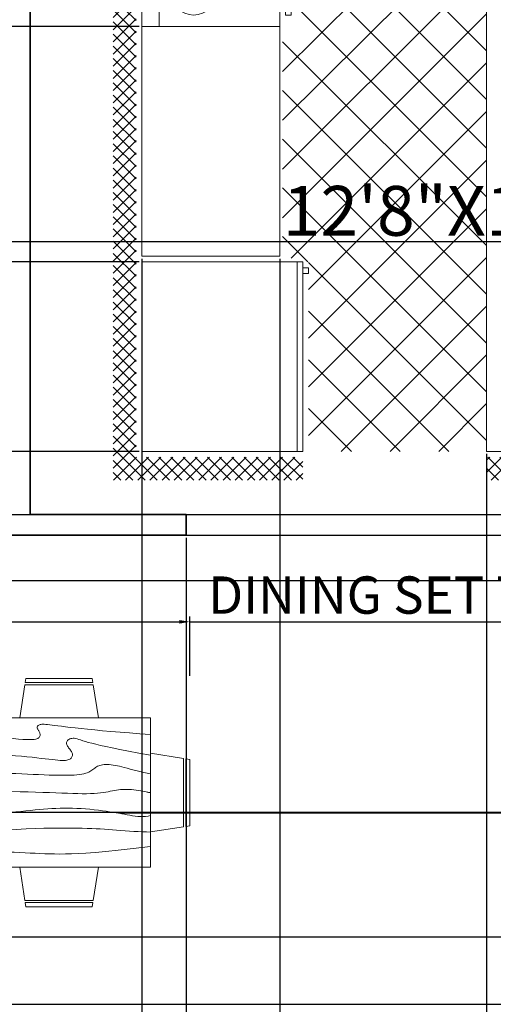
# Model space of a CAD drawing. Units: inches. Extents: x 3542 to 4275, y 1005 to 1722.
# Tile 4 of 6: x 4018 to 4132, y 1330 to 1568. Entities that reach past the tile are written whole.
import ezdxf

# ---------------------------------------------------------------- set-up
doc = ezdxf.new("R2010")
doc.units = ezdxf.units.IN
doc.layers.get('0').update_dxf_attribs({"color": 211})
for name, color, linetype, lineweight in [('A-ANNO-DIMS', 2, 'Continuous', 18), ('A-AREA-IDEN', 7, 'Continuous', 25), ('A-FLOR-FIXT', 9, 'Continuous', 18), ('A-FURN', 8, 'Continuous', 18), ('wall', 7, 'Continuous', 35)]:
    doc.layers.add(name, color=color, linetype=linetype, lineweight=lineweight)
doc.styles.get("Standard").update_dxf_attribs({"font": 'arial.ttf'})
doc.dimstyles.new('ISO-25', dxfattribs={"dimtxt": 9, "dimasz": 2.5, "dimexe": 1.25, "dimexo": 0.625, "dimtad": 1, "dimdec": 1, "dimlunit": 4, "dimtxsty": 'Standard', "dimcen": 2.5, "dimadec": 0, "dimazin": 0, "dimtfac": 1, "dimtdec": 1, "dimtmove": 0, "dimatfit": 3, "dimfxl": 1, "dimarcsym": 0})

# ---------------------------------------------------------------- blocks, each defined once
blk = doc.blocks.new('Kitchen Layout - 7 x 8 ft')
for p, q in [((-5, 81.32), (2.68, 89)), ((-5, 83.44), (0.56, 89)), ((-5, 85.56), (-1.56, 89)), ((-5, 87.68), (-3.68, 89)), ((-1, 84.97), (-5, 88.97)), ((1.09, 85), (-2.91, 89)), ((3.21, 85), (-0.79, 89)), ((0.81, 85), (4.81, 89)), ((5.34, 85), (1.34, 89)), ((2.93, 85), (6.93, 89)), ((7.46, 85), (3.46, 89)), ((5.05, 85), (9.05, 89)), ((9.58, 85), (5.58, 89)), ((7.17, 85), (11.17, 89)), ((11.7, 85), (7.7, 89)), ((9.29, 85), (13.29, 89)), ((13.82, 85), (9.82, 89)), ((11.41, 85), (15.41, 89)), ((15.94, 85), (11.94, 89)), ((13.53, 85), (17.53, 89)), ((18.06, 85), (14.06, 89)), ((15.65, 85), (19.65, 89)), ((20.18, 85), (16.18, 89)), ((17.78, 85), (21.78, 89)), ((22.31, 85), (18.31, 89)), ((19.9, 85), (23.9, 89)), ((24.43, 85), (20.43, 89)), ((22.02, 85), (26.02, 89)), ((26.55, 85), (22.55, 89)), ((24.14, 85), (28.14, 89)), ((28.67, 85), (24.67, 89)), ((26.26, 85), (30.26, 89)), ((30.79, 85), (26.79, 89)), ((28.38, 85), (32.38, 89)), ((32.91, 85), (28.91, 89)), ((30.5, 85), (34.5, 89)), ((35.03, 85), (31.03, 89)), ((32.63, 85), (36.63, 89)), ((37.16, 85), (33.16, 89)), ((34.75, 85), (38.75, 89)), ((39.28, 85), (35.28, 89)), ((36.87, 85), (40.87, 89)), ((41.4, 85), (37.4, 89)), ((38.99, 85), (42.99, 89)), ((43.52, 85), (39.52, 89)), ((41.11, 85), (45.11, 89)), ((45.64, 85), (41.64, 89)), ((43.23, 85), (47.23, 89)), ((47.76, 85), (43.76, 89)), ((45.35, 85), (49.35, 89)), ((49.88, 85), (45.88, 89)), ((47.47, 85), (51.47, 89)), ((52, 85), (48, 89)), ((49.6, 85), (53.6, 89)), ((54.13, 85), (50.13, 89)), ((51.72, 85), (55.72, 89)), ((56.25, 85), (52.25, 89)), ((53.84, 85), (57.84, 89)), ((58.37, 85), (54.37, 89)), ((55.96, 85), (59.96, 89)), ((60.49, 85), (56.49, 89)), ((58.08, 85), (62.08, 89)), ((62.61, 85), (58.61, 89)), ((60.2, 85), (64.2, 89)), ((64.73, 85), (60.73, 89)), ((62.32, 85), (66.32, 89)), ((66.85, 85), (62.85, 89)), ((64.45, 85), (68.45, 89)), ((68.97, 85), (64.97, 89)), ((66.57, 85), (70.57, 89)), ((71.1, 85), (67.1, 89)), ((68.69, 85), (72.69, 89)), ((73.22, 85), (69.22, 89)), ((70.81, 85), (74.81, 89)), ((75.34, 85), (71.34, 89)), ((72.93, 85), (76.93, 89)), ((77.46, 85), (73.46, 89)), ((75.05, 85), (79.05, 89)), ((79.58, 85), (75.58, 89)), ((77.17, 85), (81.17, 89)), ((81.7, 85), (77.7, 89)), ((79.29, 85), (83.29, 89)), ((83.82, 85), (79.82, 89)), ((81.42, 85), (85.42, 89)), ((85.95, 85), (81.95, 89)), ((83.54, 85), (87.54, 89)), ((88.07, 85), (84.07, 89)), ((85.66, 85), (89.66, 89)), ((90.19, 85), (86.19, 89)), ((87.78, 85), (91.78, 89)), ((92.31, 85), (88.31, 89)), ((89.9, 85), (93.9, 89)), ((94.43, 85), (90.43, 89)), ((92.02, 85), (96.02, 89)), ((96.55, 85), (92.55, 89)), ((94.14, 85), (98.14, 89)), ((101, 82.67), (94.67, 89)), ((96.27, 85), (100.27, 89)), ((101, 84.79), (96.79, 89)), ((97, 83.61), (101, 87.61)), ((101, 86.92), (98.92, 89)), ((-1, 82.85), (-5, 86.85)), ((-1, 80.73), (-5, 84.73)), ((97, 81.49), (101, 85.49)), ((101, 80.55), (97, 84.55)), ((-5, 79.19), (-1, 83.19)), ((-1, 78.61), (-5, 82.61)), ((34, 84), (96, 84)), ((34, 60), (34, 84)), ((96, 84), (96, 60)), ((97, 79.37), (101, 83.37)), ((101, 78.43), (97, 82.43)), ((-5, 77.07), (-1, 81.07)), ((74, 81), (95, 81)), ((97, 77.25), (101, 81.25)), ((-1, 76.49), (-5, 80.49)), ((-5, 74.95), (-1, 78.95)), ((101, 76.31), (97, 80.31)), ((97, 75.13), (101, 79.13)), ((-1, 74.36), (-5, 78.36)), ((101, 74.19), (97, 78.19)), ((-5, 72.83), (-1, 76.83)), ((-1, 72.24), (-5, 76.24)), ((97, 73.01), (101, 77.01)), ((101, 72.07), (97, 76.07)), ((-5, 70.71), (-1, 74.71)), ((-1, 70.12), (-5, 74.12)), ((97, 70.89), (101, 74.89)), ((101, 69.95), (97, 73.95)), ((-5, 68.59), (-1, 72.59)), ((97, 68.76), (101, 72.76)), ((-1, 68), (-5, 72)), ((-5, 66.47), (-1, 70.47)), ((101, 67.82), (97, 71.82)), ((97, 66.64), (101, 70.64)), ((-1, 65.88), (-5, 69.88)), ((101, 65.7), (97, 69.7)), ((-5, 64.35), (-1, 68.35)), ((-1, 63.76), (-5, 67.76)), ((97, 64.52), (101, 68.52)), ((101, 63.58), (97, 67.58)), ((-5, 62.22), (-1, 66.22)), ((-1, 61.64), (-5, 65.64)), ((97, 62.4), (101, 66.4)), ((101, 61.46), (97, 65.46)), ((-5, 60.1), (-1, 64.1)), ((-1, 59.52), (-5, 63.52)), ((97, 60.28), (101, 64.28)), ((-5, 57.98), (-1, 61.98)), ((100.34, 60), (97, 63.34)), ((98.84, 60), (101, 62.16)), ((-1, 57.39), (-5, 61.39)), ((98.22, 60), (97, 61.22)), ((100.96, 60), (101, 60.04)), ((-1.73, 56), (-5, 59.27)), ((-4.86, 56), (-1, 59.86)), ((10.4, 24), (45.9, 59.5)), ((18.88, 24), (54.38, 59.5)), ((27.37, 24), (62.87, 59.5)), ((33.03, 55.11), (37.41, 59.5)), ((96, 60), (34, 60)), ((35.85, 24), (71.35, 59.5)), ((76.2, 24), (40.7, 59.5)), ((84.68, 24), (49.18, 59.5)), ((93.17, 24), (57.67, 59.5)), ((61.31, 24), (96, 58.69)), ((96, 29.65), (66.15, 59.5)), ((80, 60), (80, 59)), ((82, 59), (82, 60)), ((87, 59), (87, 60)), ((89, 60), (89, 59)), ((-3.85, 56), (-5, 57.15)), ((-2.74, 56), (-1, 57.74)), ((0, 57), (33, 57)), ((67.71, 24), (33.68, 58.04)), ((44.34, 24), (77.84, 57.5)), ((52.82, 24), (86.32, 57.5)), ((96, 38.14), (76.64, 57.5)), ((96, 46.63), (85.13, 57.5)), ((96, 55.11), (93.57, 57.54)), ((0, 30.57), (24.43, 55)), ((0, 39.06), (15.94, 55)), ((0, 47.54), (7.46, 55)), ((1.91, 24), (32.91, 55)), ((33.77, 24), (2.77, 55)), ((42.26, 24), (11.26, 55)), ((50.74, 24), (19.74, 55)), ((59.23, 24), (28.23, 55)), ((31, 55), (31, 56)), ((32, 55), (31, 55)), ((32, 56), (32, 55)), ((69.79, 24), (96, 50.21)), ((25.29, 24), (0, 49.29)), ((78.28, 24), (96, 41.72)), ((16.8, 24), (0, 40.8)), ((86.76, 24), (96, 33.24)), ((8.32, 24), (0, 32.32)), ((95.25, 24), (96, 24.75)), ((-5, 21.92), (-2.92, 24)), ((-5, 19.8), (-1, 23.8)), ((-1, 19.21), (-5, 23.21)), ((-1, 21.33), (-3.67, 24)), ((-1, 23.45), (-1.55, 24)), ((0, 24), (96, 24)), ((0, 0), (0, 24)), ((96, 24), (96, 0)), ((97, 22.1), (98.9, 24)), ((97, 19.97), (101, 23.97)), ((101, 19.03), (97, 23.03)), ((101, 21.16), (98.16, 24)), ((101, 23.28), (100.28, 24)), ((-5, 17.68), (-1, 21.68)), ((-1, 17.09), (-5, 21.09)), ((97, 17.85), (101, 21.85)), ((101, 16.91), (97, 20.91)), ((-5, 15.55), (-1, 19.55)), ((-1, 14.97), (-5, 18.97)), ((97, 15.73), (101, 19.73)), ((-5, 13.43), (-1, 17.43)), ((47.25, 6.5), (47.25, 18.5)), ((48.75, 18.5), (48.75, 6.5)), ((101, 14.79), (97, 18.79)), ((97, 13.61), (101, 17.61)), ((-1, 12.85), (-5, 16.85)), ((101, 12.67), (97, 16.67)), ((97, 11.49), (101, 15.49)), ((-5, 11.31), (-1, 15.31)), ((-1, 10.73), (-5, 14.73)), ((101, 10.55), (97, 14.55)), ((-5, 9.19), (-1, 13.19)), ((-1, 8.6), (-5, 12.6)), ((97, 9.37), (101, 13.37)), ((101, 8.43), (97, 12.43)), ((-5, 7.07), (-1, 11.07)), ((-1, 6.48), (-5, 10.48)), ((97, 7.25), (101, 11.25)), ((101, 6.31), (97, 10.31)), ((-5, 4.95), (-1, 8.95)), ((97, 5.12), (101, 9.12)), ((-1, 4.36), (-5, 8.36)), ((101, 4.18), (97, 8.18)), ((97, 3), (101, 7)), ((-5, 2.83), (-1, 6.83)), ((-1, 2.24), (-5, 6.24)), ((101, 2.06), (97, 6.06)), ((-5, 0.71), (-1, 4.71)), ((-1, 0.12), (-5, 4.12)), ((64, 4), (32, 4)), ((97, 0.88), (101, 4.88)), ((101, -0.06), (97, 3.94)), ((-5, -1.42), (-1, 2.58)), ((2, -5), (-5, 2)), ((93.24, -5), (101, 2.76)), ((101, -2.18), (97, 1.82)), ((-5, -3.54), (-1, 0.46)), ((96, 0), (0, 0)), ((95.36, -5), (101, 0.64)), ((-0.12, -5), (-5, -0.12)), ((-4.34, -5), (-0.34, -1)), ((-2.22, -5), (1.78, -1)), ((-0.1, -5), (3.9, -1)), ((4.12, -5), (0.12, -1)), ((2.02, -5), (6.02, -1)), ((6.24, -5), (2.24, -1)), ((4.14, -5), (8.14, -1)), ((8.36, -5), (4.36, -1)), ((6.27, -5), (10.27, -1)), ((10.48, -5), (6.48, -1)), ((8.39, -5), (12.39, -1)), ((12.6, -5), (8.6, -1)), ((10.51, -5), (14.51, -1)), ((14.73, -5), (10.73, -1)), ((12.63, -5), (16.63, -1)), ((16.85, -5), (12.85, -1)), ((14.75, -5), (18.75, -1)), ((18.97, -5), (14.97, -1)), ((16.87, -5), (20.87, -1)), ((21.09, -5), (17.09, -1)), ((18.99, -5), (22.99, -1)), ((23.21, -5), (19.21, -1)), ((21.11, -5), (25.11, -1)), ((25.33, -5), (21.33, -1)), ((23.24, -5), (27.24, -1)), ((27.45, -5), (23.45, -1)), ((25.36, -5), (29.36, -1)), ((29.57, -5), (25.57, -1)), ((30, -3.3), (27.7, -1)), ((30, -1.18), (29.82, -1)), ((66, -2.54), (67.54, -1)), ((66, -4.66), (69.66, -1)), ((69.88, -5), (66, -1.12)), ((67.78, -5), (71.78, -1)), ((72, -5), (68, -1)), ((69.9, -5), (73.9, -1)), ((74.12, -5), (70.12, -1)), ((72.03, -5), (76.03, -1)), ((76.24, -5), (72.24, -1)), ((74.15, -5), (78.15, -1)), ((78.36, -5), (74.36, -1)), ((76.27, -5), (80.27, -1)), ((80.49, -5), (76.49, -1)), ((78.39, -5), (82.39, -1)), ((82.61, -5), (78.61, -1)), ((80.51, -5), (84.51, -1)), ((84.73, -5), (80.73, -1)), ((82.63, -5), (86.63, -1)), ((86.85, -5), (82.85, -1)), ((84.75, -5), (88.75, -1)), ((88.97, -5), (84.97, -1)), ((86.88, -5), (90.88, -1)), ((91.09, -5), (87.09, -1)), ((89, -5), (93, -1)), ((93.21, -5), (89.21, -1)), ((91.12, -5), (95.12, -1)), ((95.34, -5), (91.34, -1)), ((97.46, -5), (93.46, -1)), ((99.58, -5), (95.58, -1)), ((101, -4.3), (97, -0.3)), ((97.48, -5), (101, -1.48)), ((-2.25, -5), (-5, -2.25)), ((27.48, -5), (30, -2.48)), ((67.76, -5), (66, -3.24)), ((-4.37, -5), (-5, -4.37)), ((29.6, -5), (30, -4.6)), ((99.6, -5), (101, -3.6))]:
    blk.add_line(p, q)
for points in [[(0, 56), (0, 84), (33, 84), (33, 56)], [(74, 60), (74, 84), (95, 84), (95, 60)], [(76, 58), (76, 59), (93, 59), (93, 58)]]:
    blk.add_lwpolyline(points, close=True)
for points in [[(33.5, 21), (62.5, 21)], [(32, 1.5), (32, 19.5)], [(34.5, 19.5), (46.25, 19.5)], [(49.75, 19.5), (61.5, 19.5)], [(64, 19.5), (64, 1.5)], [(33.5, 6.5), (33.5, 18.5)], [(62.5, 18.5), (62.5, 6.5)], [(46.25, 5.5), (34.5, 5.5)], [(61.5, 5.5), (49.75, 5.5)], [(62.5, 0), (33.5, 0)]]:
    blk.add_lwpolyline(points)
for centre, radius in [((80, 75), 4), ((80, 75), 3), ((89, 75), 3), ((80, 75), 2), ((80, 75), 1), ((89, 75), 2), ((89, 75), 1), ((80, 66), 3), ((89, 66), 4), ((89, 66), 3), ((80, 66), 2), ((80, 66), 1), ((89, 66), 2), ((89, 66), 1), ((40.5, 12.5), 1), ((40.5, 12.5), 0.5), ((55.5, 12.5), 1), ((55.5, 12.5), 0.5)]:
    blk.add_circle(centre, radius)
for centre, radius, start, end in [((33.5, 19.5), 1.5, 90, 180), ((62.5, 19.5), 1.5, 0, 90), ((34.5, 18.5), 1, 90, 180), ((46.25, 18.5), 1, 0, 90), ((49.75, 18.5), 1, 90, 180), ((61.5, 18.5), 1, 0, 90), ((34.5, 6.5), 1, 180, 270), ((46.25, 6.5), 1, 270, 0), ((49.75, 6.5), 1, 180, 270), ((61.5, 6.5), 1, 270, 0), ((33.5, 1.5), 1.5, 180, 270), ((62.5, 1.5), 1.5, 270, 0)]:
    blk.add_arc(centre, radius, start, end)
blk = doc.blocks.new('Dining Set - 36 x 72 in.')
for p, q in [((-22, 27.5), (-22.1562, 26.50042)), ((-5.8416, 26.5), (-22.1534, 26.5)), ((-22, 27.5), (-6, 27.5)), ((-5.8437, 26.49966), (-6, 27.5)), ((6, 27.5), (5.8438, 26.50042)), ((22.1584, 26.5), (5.8466, 26.5)), ((6, 27.5), (22, 27.5)), ((22.1563, 26.49966), (22, 27.5)), ((-22.2343, 26.00059), (-23.4847, 17.99762)), ((-22.2304, 26), (-5.7608, 26)), ((-4.5152, 17.99762), (-5.7655, 25.99926)), ((5.7657, 26.00059), (4.5153, 17.99762)), ((5.7696, 26), (22.2392, 26)), ((23.4848, 17.99762), (22.2345, 25.99926)), ((36, 18), (-36, 18)), ((-36, 18), (-36, -18)), ((36, -18), (36, 18)), ((-45.5, 8), (-44.5004, 8.15617)), ((-45.5, 8), (-45.5, -8)), ((-44.5, -8.15843), (-44.5, 8.15338)), ((-44.0006, 8.23428), (-35.9976, 9.48474)), ((-44, 8.23041), (-44, -8.23915)), ((44.0006, 8.23428), (35.9976, 9.48474)), ((44, 8.23041), (44, -8.23915)), ((44.5, -8.15843), (44.5, 8.15338)), ((45.5, 8), (44.5005, 8.15617)), ((45.5, 8), (45.5, -8)), ((-44.4997, -8.15631), (-45.5, -8)), ((-35.9976, -9.48476), (-43.9993, -8.2345)), ((35.9976, -9.48476), (43.9993, -8.2345)), ((44.4997, -8.15631), (45.5, -8)), ((-36, -18), (36, -18)), ((-22.2343, -26.0006), (-23.4847, -17.99762)), ((-4.5152, -17.99762), (-5.7655, -25.99928)), ((5.7657, -26.0006), (4.5153, -17.99762)), ((23.4848, -17.99762), (22.2345, -25.99928)), ((-22.2304, -26), (-5.7608, -26)), ((5.7696, -26), (22.2392, -26)), ((-22, -27.5), (-22.1562, -26.50044)), ((-5.8416, -26.5), (-22.1534, -26.5)), ((-22, -27.5), (-6, -27.5)), ((-5.8437, -26.49967), (-6, -27.5)), ((6, -27.5), (5.8438, -26.50044)), ((22.1584, -26.5), (5.8466, -26.5)), ((6, -27.5), (22, -27.5)), ((22.1563, -26.49967), (22, -27.5))]:
    blk.add_line(p, q)
for points in [[(-36, 15), (-31.1772, 14.97754), (-26.8079, 14.91406), (-22.8538, 14.81543), (-19.276, 14.6875), (-16.0362, 14.53613), (-13.0957, 14.36718), (-10.4159, 14.18652), (-7.9583, 14), (-5.6904, 13.81315), (-3.6035, 13.63021), (-1.6954, 13.45508), (0.0365, 13.29166), (1.5945, 13.14388), (2.9811, 13.01562), (4.1988, 12.9108), (5.25, 12.83333), (6.1393, 12.78613), (6.8802, 12.76823), (7.4883, 12.77767), (7.9792, 12.8125), (8.3685, 12.87077), (8.6719, 12.95052), (8.9049, 13.0498), (9.0833, 13.16666), (9.2205, 13.29899), (9.3216, 13.44401), (9.3895, 13.59879), (9.4271, 13.76041), (9.4373, 13.92594), (9.4232, 14.09245), (9.3875, 14.257), (9.3333, 14.41666), (9.2638, 14.56917), (9.1836, 14.71484), (9.0975, 14.85465), (9.0104, 14.98958), (8.9272, 15.1206), (8.8529, 15.2487), (8.7922, 15.37483), (8.75, 15.5), (8.7305, 15.62467), (8.7344, 15.74739), (8.7617, 15.86621), (8.8125, 15.97916), (8.8867, 16.08431), (8.9844, 16.17968), (9.1055, 16.26334), (9.25, 16.33333), (9.4189, 16.38802), (9.6172, 16.42708), (9.8506, 16.45052), (10.125, 16.45833), (10.4463, 16.45052), (10.8203, 16.42708), (11.2529, 16.38802), (11.75, 16.33333), (12.3184, 16.26318), (12.9694, 16.17838), (13.7151, 16.07991), (14.5677, 15.96875), (15.5395, 15.84586), (16.6426, 15.71224), (17.8893, 15.56884), (19.2917, 15.41666), (20.859, 15.25667), (22.5879, 15.08984), (24.4721, 14.91715), (26.5052, 14.73958), (28.6809, 14.5581), (30.9929, 14.3737), (33.4347, 14.18733), (36, 14)], [(-36, 10), (-28.9766, 10.14274), (-23.1725, 10.20442), (-18.4241, 10.19775), (-14.5677, 10.13541), (-11.4399, 10.03011), (-8.877, 9.89453), (-6.7154, 9.74137), (-4.7917, 9.58333), (-2.9698, 9.43082), (-1.2246, 9.28515), (0.4415, 9.14534), (2.026, 9.01041), (3.5266, 8.87939), (4.9408, 8.7513), (6.266, 8.62516), (7.5, 8.5), (8.6411, 8.37549), (9.6914, 8.2539), (10.6538, 8.13818), (11.5312, 8.03125), (12.3267, 7.93603), (13.043, 7.85547), (13.6831, 7.79248), (14.25, 7.75), (14.7471, 7.7303), (15.1797, 7.73307), (15.5537, 7.75732), (15.875, 7.80208), (16.1494, 7.86637), (16.3828, 7.94922), (16.5811, 8.04964), (16.75, 8.16666), (16.8944, 8.29915), (17.0143, 8.44531), (17.1089, 8.60319), (17.1771, 8.77083), (17.218, 8.94629), (17.2305, 9.1276), (17.2137, 9.31282), (17.1667, 9.5), (17.0895, 9.6875), (16.987, 9.875), (16.8649, 10.0625), (16.7292, 10.25), (16.5856, 10.4375), (16.4401, 10.625), (16.2985, 10.8125), (16.1667, 11), (16.05, 11.18733), (15.9518, 11.3737), (15.8752, 11.5581), (15.8229, 11.73958), (15.798, 11.91715), (15.8034, 12.08984), (15.842, 12.25667), (15.9167, 12.41666), (16.0295, 12.56836), (16.1784, 12.70833), (16.3605, 12.83268), (16.5729, 12.9375), (16.8127, 13.01888), (17.0768, 13.07291), (17.3625, 13.0957), (17.6667, 13.08333), (17.9894, 13.03312), (18.3418, 12.94726), (18.7382, 12.82918), (19.1927, 12.68229), (19.7195, 12.51001), (20.3327, 12.31575), (21.0465, 12.10294), (21.875, 11.875), (22.8357, 11.63354), (23.959, 11.37304), (25.2786, 11.08618), (26.8282, 10.76562), (28.6414, 10.40405), (30.752, 9.99414), (33.1936, 9.52856), (36, 9)], [(-36, 5.5), (-30.7157, 5.3348), (-26.069, 5.20963), (-21.9946, 5.11767), (-18.4271, 5.05208), (-15.3009, 5.00602), (-12.5508, 4.97265), (-10.1112, 4.94515), (-7.9167, 4.91666), (-5.909, 4.88167), (-4.0586, 4.83984), (-2.3429, 4.79215), (-0.7396, 4.73958), (0.7739, 4.6831), (2.22, 4.6237), (3.6213, 4.56233), (5, 4.5), (6.373, 4.43782), (7.7344, 4.3776), (9.0723, 4.32129), (10.375, 4.27083), (11.6309, 4.22819), (12.8281, 4.19531), (13.9551, 4.17415), (15, 4.16666), (15.954, 4.17448), (16.819, 4.19791), (17.6001, 4.23698), (18.3021, 4.29166), (18.9299, 4.36198), (19.4883, 4.44791), (19.9823, 4.54948), (20.4167, 4.66666), (20.7969, 4.79899), (21.1302, 4.94401), (21.4245, 5.09879), (21.6875, 5.26041), (21.9271, 5.42594), (22.1511, 5.59245), (22.3672, 5.757), (22.5834, 5.91666), (22.8065, 6.06868), (23.0404, 6.21093), (23.2879, 6.34147), (23.5521, 6.45833), (23.8358, 6.55957), (24.142, 6.64323), (24.4735, 6.70735), (24.8334, 6.75), (25.2235, 6.76969), (25.642, 6.76692), (26.0858, 6.74267), (26.5521, 6.69791), (27.0379, 6.63362), (27.5404, 6.55078), (28.0565, 6.45036), (28.5834, 6.33333), (29.1242, 6.19987), (29.7071, 6.04687), (30.3661, 5.87044), (31.1354, 5.66666), (32.0493, 5.43164), (33.142, 5.16146), (34.4475, 4.85221), (36, 4.5)], [(-36, -1), (-30.7915, -0.6591), (-26.0195, -0.38216), (-21.6519, -0.16284), (-17.6563, 0.00521), (-14.0005, 0.12833), (-10.6523, 0.21289), (-7.5796, 0.26522), (-4.75, 0.29166), (-2.134, 0.29793), (0.2878, 0.28711), (2.5317, 0.26163), (4.6146, 0.22396), (6.5529, 0.17651), (8.3633, 0.12174), (10.0623, 0.06209), (11.6667, 0), (13.1899, -0.06201), (14.6341, -0.1211), (15.9982, -0.17432), (17.2813, -0.21875), (18.4823, -0.25147), (19.6003, -0.26953), (20.6343, -0.27002), (21.5834, -0.25), (22.4481, -0.20768), (23.2357, -0.14584), (23.9549, -0.06836), (24.6146, 0.02083), (25.2235, 0.11784), (25.7904, 0.21875), (26.3241, 0.31966), (26.8334, 0.41666), (27.3265, 0.50618), (27.8099, 0.58593), (28.2894, 0.65397), (28.7709, 0.70833), (29.2601, 0.74707), (29.763, 0.76823), (30.2855, 0.76985), (30.8334, 0.75), (31.4088, 0.70784), (31.9994, 0.64713), (32.589, 0.57275), (33.1615, 0.48958), (33.7008, 0.4025), (34.1908, 0.3164), (34.6153, 0.23616), (34.9584, 0.16666), (35.2099, 0.11165), (35.3848, 0.07031), (35.504, 0.04069), (35.5886, 0.02083), (35.6594, 0.00879), (35.7377, 0.0026), (35.8442, 0.00032), (36, 0)], [(-36, -6.5), (-27.1843, -6.31267), (-20.084, -6.1263), (-14.469, -5.9419), (-10.1094, -5.76042), (-6.7752, -5.58285), (-4.2363, -5.41016), (-2.2629, -5.24333), (-0.625, -5.08334), (0.8708, -4.93099), (2.2715, -4.78646), (3.5872, -4.64974), (4.8281, -4.52084), (6.0046, -4.39974), (7.127, -4.28646), (8.2053, -4.18099), (9.25, -4.08334), (10.2705, -3.99382), (11.2734, -3.91407), (12.2647, -3.84603), (13.25, -3.79167), (14.2354, -3.75293), (15.2266, -3.73177), (16.2295, -3.73015), (17.25, -3.75), (18.2912, -3.79248), (19.3451, -3.85547), (20.4009, -3.93604), (21.4479, -4.03125), (22.4754, -4.13819), (23.4727, -4.25391), (24.4289, -4.37549), (25.3334, -4.5), (26.1785, -4.62492), (26.9694, -4.74935), (27.7145, -4.87281), (28.4219, -4.99479), (29.1, -5.11483), (29.7572, -5.23242), (30.4016, -5.34709), (31.0417, -5.45834), (31.6837, -5.56437), (32.3262, -5.65821), (32.9658, -5.73153), (33.599, -5.77604), (34.2224, -5.78345), (34.8327, -5.74545), (35.4264, -5.65373), (36, -5.5)], [(-36, -10), (-26.4022, -9.81299), (-18.4675, -9.62891), (-11.9839, -9.45069), (-6.7396, -9.28125), (-2.5226, -9.12354), (0.8789, -8.98047), (3.6769, -8.85498), (6.0833, -8.75), (8.2767, -8.66765), (10.3021, -8.60677), (12.1712, -8.56543), (13.8958, -8.54167), (15.4876, -8.53353), (16.9583, -8.53907), (18.3197, -8.55632), (19.5834, -8.58334), (20.7616, -8.61841), (21.8685, -8.66081), (22.9188, -8.71004), (23.9271, -8.76563), (24.9081, -8.82707), (25.8763, -8.89388), (26.8465, -8.96558), (27.8334, -9.04167), (28.8474, -9.12118), (29.8828, -9.20117), (30.93, -9.27824), (31.9792, -9.34896), (33.0205, -9.40991), (34.0443, -9.45768), (35.0407, -9.48885), (36, -9.5)], [(-36, -14.5), (-30.0881, -14.33513), (-25.0332, -14.21224), (-20.7312, -14.12647), (-17.0781, -14.07292), (-13.97, -14.04671), (-11.3027, -14.04297), (-8.9724, -14.05681), (-6.875, -14.08334), (-4.9224, -14.11833), (-3.0905, -14.16016), (-1.3709, -14.20785), (0.2448, -14.26042), (1.7647, -14.3169), (3.1973, -14.3763), (4.5507, -14.43767), (5.8333, -14.5), (7.0554, -14.5621), (8.235, -14.62175), (9.3922, -14.67652), (10.5469, -14.72396), (11.7192, -14.76164), (12.929, -14.78711), (14.1965, -14.79794), (15.5417, -14.79167), (16.9933, -14.76424), (18.6152, -14.70508), (20.4804, -14.60197), (22.6615, -14.44271), (25.2312, -14.21509), (28.2624, -13.9069), (31.8277, -13.50594), (36, -13)]]:
    blk.add_lwpolyline(points)
blk = doc.blocks.new('*D31')
at = {"layer": 'A-ANNO-DIMS', "color": 0, "lineweight": -2, "transparency": 16777216}
for p, q in [((3968.37, 1409.56), (3968.37, 1423.84)), ((4059.37, 1409.56), (4059.37, 1423.84)), ((3970.87, 1422.59), (4056.87, 1422.59)), ((4059.37, 1422.59), (4162.04, 1422.59))]:
    blk.add_line(p, q, dxfattribs=at)
at = {"layer": 'A-ANNO-DIMS', "color": 0, "transparency": 16777216}
for points in [[(3970.87, 1423.01), (3970.87, 1422.17), (3968.37, 1422.59)], [(4056.87, 1423.01), (4056.87, 1422.17), (4059.37, 1422.59)]]:
    blk.add_solid(points, dxfattribs=at)
at = {"layer": 'Defpoints', "color": 0, "transparency": 16777216}
for p in [(4059.37, 1422.59), (3968.37, 1408.94), (4059.37, 1408.94)]:
    blk.add_point(p, dxfattribs=at)
at = {"layer": 'A-ANNO-DIMS', "color": 0, "transparency": 16777216, "insert": (4111.95, 1427.87), "char_height": 9, "attachment_point": 5}
blk.add_mtext('DINING SET 7\'-7"', dxfattribs=at)
blk = doc.blocks.new('*D49')
at = {"layer": 'A-ANNO-DIMS', "color": 0, "lineweight": -2, "transparency": 16777216}
for p, q in [((4058.5, 1442.8), (4058.5, 1099.93)), ((4140.16, 1442.8), (4140.16, 1099.93)), ((4061, 1101.18), (4137.66, 1101.18))]:
    blk.add_line(p, q, dxfattribs=at)
at = {"layer": 'A-ANNO-DIMS', "color": 0, "transparency": 16777216}
for points in [[(4061, 1101.59), (4061, 1100.76), (4058.5, 1101.18)], [(4137.66, 1101.59), (4137.66, 1100.76), (4140.16, 1101.18)]]:
    blk.add_solid(points, dxfattribs=at)
at = {"layer": 'Defpoints', "color": 0, "transparency": 16777216}
for p in [(4058.5, 1443.43), (4140.16, 1443.43), (4140.16, 1101.18)]:
    blk.add_point(p, dxfattribs=at)
at = {"layer": 'A-ANNO-DIMS', "color": 0, "transparency": 16777216, "insert": (4099.33, 1106.46), "char_height": 9, "attachment_point": 5}
blk.add_mtext('6\'-9 1/2"', dxfattribs=at)
blk = doc.blocks.new('*D51')
at = {"layer": 'A-ANNO-DIMS', "color": 0, "lineweight": -2, "transparency": 16777216}
for p, q in [((4047.82, 1510.06), (4047.82, 1099.93)), ((4081.03, 1510.06), (4081.03, 1099.93)), ((4050.32, 1101.18), (4078.53, 1101.18))]:
    blk.add_line(p, q, dxfattribs=at)
at = {"layer": 'A-ANNO-DIMS', "color": 0, "transparency": 16777216}
for points in [[(4050.32, 1101.59), (4050.32, 1100.76), (4047.82, 1101.18)], [(4078.53, 1101.59), (4078.53, 1100.76), (4081.03, 1101.18)]]:
    blk.add_solid(points, dxfattribs=at)
at = {"layer": 'Defpoints', "color": 0, "transparency": 16777216}
for p in [(4047.82, 1510.69), (4081.03, 1510.69), (4081.03, 1101.18)]:
    blk.add_point(p, dxfattribs=at)
at = {"layer": 'A-ANNO-DIMS', "color": 0, "transparency": 16777216, "insert": (4064.42, 1106.4), "char_height": 9, "attachment_point": 5}
blk.add_mtext('2\'-9"', dxfattribs=at)
blk = doc.blocks.new('*D52')
at = {"layer": 'A-ANNO-DIMS', "color": 0, "lineweight": -2, "transparency": 16777216}
for p, q in [((4081.03, 1510.06), (4081.03, 1099.93)), ((4130.83, 1463.03), (4130.83, 1099.93)), ((4083.53, 1101.18), (4128.33, 1101.18))]:
    blk.add_line(p, q, dxfattribs=at)
at = {"layer": 'A-ANNO-DIMS', "color": 0, "transparency": 16777216}
for points in [[(4083.53, 1101.59), (4083.53, 1100.76), (4081.03, 1101.18)], [(4128.33, 1101.59), (4128.33, 1100.76), (4130.83, 1101.18)]]:
    blk.add_solid(points, dxfattribs=at)
at = {"layer": 'Defpoints', "color": 0, "transparency": 16777216}
for p in [(4081.03, 1510.69), (4130.83, 1463.65), (4130.83, 1101.18)]:
    blk.add_point(p, dxfattribs=at)
at = {"layer": 'A-ANNO-DIMS', "color": 0, "transparency": 16777216, "insert": (4105.93, 1106.32), "char_height": 9, "attachment_point": 5}
blk.add_mtext('4\'-2"', dxfattribs=at)
blk = doc.blocks.new('*D53')
at = {"layer": 'A-ANNO-DIMS', "color": 0, "lineweight": -2, "transparency": 16777216}
for p, q in [((4130.83, 1463.03), (4130.83, 1099.93)), ((4164.03, 1463.03), (4164.03, 1099.93)), ((4133.33, 1101.18), (4161.53, 1101.18))]:
    blk.add_line(p, q, dxfattribs=at)
at = {"layer": 'A-ANNO-DIMS', "color": 0, "transparency": 16777216}
for points in [[(4133.33, 1101.59), (4133.33, 1100.76), (4130.83, 1101.18)], [(4161.53, 1101.59), (4161.53, 1100.76), (4164.03, 1101.18)]]:
    blk.add_solid(points, dxfattribs=at)
at = {"layer": 'Defpoints', "color": 0, "transparency": 16777216}
for p in [(4130.83, 1463.65), (4164.03, 1463.65), (4164.03, 1101.18)]:
    blk.add_point(p, dxfattribs=at)
at = {"layer": 'A-ANNO-DIMS', "color": 0, "transparency": 16777216, "insert": (4147.43, 1106.4), "char_height": 9, "attachment_point": 5}
blk.add_mtext('2\'-9"', dxfattribs=at)
blk = doc.blocks.new('*D54')
at = {"layer": 'A-ANNO-DIMS', "color": 0, "lineweight": -2, "transparency": 16777216}
for p, q in [((4047.2, 1596.46), (3559.02, 1596.46)), ((3560.27, 1593.96), (3560.27, 1568.52)), ((4047.2, 1566.02), (3559.02, 1566.02)), ((3560.27, 1566.02), (3560.27, 1517.22))]:
    blk.add_line(p, q, dxfattribs=at)
at = {"layer": 'A-ANNO-DIMS', "color": 0, "transparency": 16777216}
for points in [[(3559.85, 1593.96), (3560.69, 1593.96), (3560.27, 1596.46)], [(3559.85, 1568.52), (3560.69, 1568.52), (3560.27, 1566.02)]]:
    blk.add_solid(points, dxfattribs=at)
at = {"layer": 'Defpoints', "color": 0, "transparency": 16777216}
for p in [(4047.82, 1596.46), (3560.27, 1566.02), (4047.82, 1566.02)]:
    blk.add_point(p, dxfattribs=at)
at = {"layer": 'A-ANNO-DIMS', "color": 0, "transparency": 16777216, "insert": (3554.99, 1540.37), "char_height": 9, "attachment_point": 5, "rotation": 90}
blk.add_mtext('2\'-6 1/2"', dxfattribs=at)
blk = doc.blocks.new('*D55')
at = {"layer": 'A-ANNO-DIMS', "color": 0, "lineweight": -2, "transparency": 16777216}
for p, q in [((3560.27, 1509.3), (3560.27, 1557.94)), ((4047.2, 1509.3), (3559.02, 1509.3)), ((3560.27, 1466.15), (3560.27, 1506.8)), ((4047.2, 1463.65), (3559.02, 1463.65))]:
    blk.add_line(p, q, dxfattribs=at)
at = {"layer": 'A-ANNO-DIMS', "color": 0, "transparency": 16777216}
for points in [[(3559.85, 1506.8), (3560.69, 1506.8), (3560.27, 1509.3)], [(3559.85, 1466.15), (3560.69, 1466.15), (3560.27, 1463.65)]]:
    blk.add_solid(points, dxfattribs=at)
at = {"layer": 'Defpoints', "color": 0, "transparency": 16777216}
for p in [(3560.27, 1509.3), (4047.82, 1509.3), (4047.82, 1463.65)]:
    blk.add_point(p, dxfattribs=at)
at = {"layer": 'A-ANNO-DIMS', "color": 0, "transparency": 16777216, "insert": (3554.99, 1534.87), "char_height": 9, "attachment_point": 5, "rotation": 90}
blk.add_mtext('3\'-9 1/2"', dxfattribs=at)
blk = doc.blocks.new('*D64')
at = {"layer": 'A-ANNO-DIMS', "color": 0, "lineweight": -2, "transparency": 16777216}
for p, q in [((3741.01, 1376.72), (4214.39, 1376.72)), ((4213.14, 1374.22), (4213.14, 1349.22)), ((3741.01, 1346.72), (4214.39, 1346.72))]:
    blk.add_line(p, q, dxfattribs=at)
at = {"layer": 'A-ANNO-DIMS', "color": 0, "transparency": 16777216}
for points in [[(4212.72, 1374.22), (4213.56, 1374.22), (4213.14, 1376.72)], [(4212.72, 1349.22), (4213.56, 1349.22), (4213.14, 1346.72)]]:
    blk.add_solid(points, dxfattribs=at)
at = {"layer": 'Defpoints', "color": 0, "transparency": 16777216}
for p in [(3740.38, 1376.72), (3740.38, 1346.72), (4213.14, 1346.72)]:
    blk.add_point(p, dxfattribs=at)
at = {"layer": 'A-ANNO-DIMS', "color": 0, "transparency": 16777216, "insert": (4207.92, 1361.72), "char_height": 9, "attachment_point": 5, "rotation": 90}
blk.add_mtext('2\'-6"', dxfattribs=at)
blk = doc.blocks.new('*D66')
at = {"layer": 'A-ANNO-DIMS', "color": 0, "lineweight": -2, "transparency": 16777216}
for p, q in [((3735.51, 1443.43), (4214.39, 1443.43)), ((4213.14, 1440.93), (4213.14, 1435.03)), ((3735.95, 1432.53), (4214.39, 1432.53)), ((4213.14, 1432.53), (4213.14, 1397.86))]:
    blk.add_line(p, q, dxfattribs=at)
at = {"layer": 'A-ANNO-DIMS', "color": 0, "transparency": 16777216}
for points in [[(4212.72, 1440.93), (4213.56, 1440.93), (4213.14, 1443.43)], [(4212.72, 1435.03), (4213.56, 1435.03), (4213.14, 1432.53)]]:
    blk.add_solid(points, dxfattribs=at)
at = {"layer": 'Defpoints', "color": 0, "transparency": 16777216}
for p in [(3734.89, 1443.43), (3735.32, 1432.53), (4213.14, 1432.53)]:
    blk.add_point(p, dxfattribs=at)
at = {"layer": 'A-ANNO-DIMS', "color": 0, "transparency": 16777216, "insert": (4207.92, 1413.94), "char_height": 9, "attachment_point": 5, "rotation": 90}
blk.add_mtext('0\'-11"', dxfattribs=at)
blk = doc.blocks.new('*D67')
at = {"layer": 'A-ANNO-DIMS', "color": 0, "lineweight": -2, "transparency": 16777216}
for p, q in [((4213.14, 1346.72), (4213.14, 1394.52)), ((3741.01, 1346.72), (4214.39, 1346.72)), ((4213.14, 1332.93), (4213.14, 1344.22)), ((3740.51, 1330.43), (4214.39, 1330.43))]:
    blk.add_line(p, q, dxfattribs=at)
at = {"layer": 'A-ANNO-DIMS', "color": 0, "transparency": 16777216}
for points in [[(4212.72, 1344.22), (4213.56, 1344.22), (4213.14, 1346.72)], [(4212.72, 1332.93), (4213.56, 1332.93), (4213.14, 1330.43)]]:
    blk.add_solid(points, dxfattribs=at)
at = {"layer": 'Defpoints', "color": 0, "transparency": 16777216}
for p in [(3740.38, 1346.72), (4213.14, 1346.72), (3739.89, 1330.43)]:
    blk.add_point(p, dxfattribs=at)
at = {"layer": 'A-ANNO-DIMS', "color": 0, "transparency": 16777216, "insert": (4207.86, 1371.87), "char_height": 9, "attachment_point": 5, "rotation": 90}
blk.add_mtext('1\'-4 1/2"', dxfattribs=at)
blk = doc.blocks.new('*D73')
at = {"layer": 'A-ANNO-DIMS', "color": 0, "lineweight": -2, "transparency": 16777216}
for p, q in [((3836.51, 1514.23), (4214.39, 1514.23)), ((4213.14, 1450.93), (4213.14, 1511.73)), ((3836.51, 1448.43), (4214.39, 1448.43))]:
    blk.add_line(p, q, dxfattribs=at)
at = {"layer": 'A-ANNO-DIMS', "color": 0, "transparency": 16777216}
for points in [[(4212.72, 1511.73), (4213.56, 1511.73), (4213.14, 1514.23)], [(4212.72, 1450.93), (4213.56, 1450.93), (4213.14, 1448.43)]]:
    blk.add_solid(points, dxfattribs=at)
at = {"layer": 'Defpoints', "color": 0, "transparency": 16777216}
for p in [(3835.89, 1514.23), (4213.14, 1514.23), (3835.89, 1448.43)]:
    blk.add_point(p, dxfattribs=at)
at = {"layer": 'A-ANNO-DIMS', "color": 0, "transparency": 16777216, "insert": (4207.92, 1481.33), "char_height": 9, "attachment_point": 5, "rotation": 90}
blk.add_mtext('5\'-6"', dxfattribs=at)
blk = doc.blocks.new('*D74')
at = {"layer": 'A-ANNO-DIMS', "color": 0, "lineweight": -2, "transparency": 16777216}
for p, q in [((4042.19, 1376.59), (4163.39, 1376.59)), ((4266.24, 1376.59), (4165.89, 1376.59))]:
    blk.add_line(p, q, dxfattribs=at)
at = {"layer": 'A-ANNO-DIMS', "color": 0, "transparency": 16777216}
blk.add_solid([(4165.89, 1377.01), (4165.89, 1376.18), (4163.39, 1376.59)], dxfattribs=at)
at = {"layer": 'Defpoints', "color": 0, "transparency": 16777216}
for p in [(4042.19, 1376.59), (4163.39, 1376.59)]:
    blk.add_point(p, dxfattribs=at)
at = {"layer": 'A-ANNO-DIMS', "color": 0, "transparency": 16777216, "insert": (4236.11, 1381.81), "char_height": 9, "attachment_point": 5, "rotation": 359.9999}
blk.add_mtext('2X R10\'-1"', dxfattribs=at)
blk = doc.blocks.new('*D75')
at = {"layer": 'A-ANNO-DIMS', "color": 0, "lineweight": -2, "transparency": 16777216}
for p, q in [((4055.14, 1376.59), (4169.39, 1376.59)), ((4275.07, 1376.59), (4171.89, 1376.59))]:
    blk.add_line(p, q, dxfattribs=at)
at = {"layer": 'A-ANNO-DIMS', "color": 0, "transparency": 16777216}
blk.add_solid([(4171.89, 1377.01), (4171.89, 1376.18), (4169.39, 1376.59)], dxfattribs=at)
at = {"layer": 'Defpoints', "color": 0, "transparency": 16777216}
for p in [(4055.14, 1376.59), (4169.39, 1376.59)]:
    blk.add_point(p, dxfattribs=at)
at = {"layer": 'A-ANNO-DIMS', "color": 0, "transparency": 16777216, "insert": (4237.94, 1381.87), "char_height": 9, "attachment_point": 5, "rotation": 359.9999}
blk.add_mtext('2X R9\'-6 1/2"', dxfattribs=at)

msp = doc.modelspace()

# ---------------------------------------------------------------- linework, layer by layer
at = {"layer": 'wall'}
for p, q in [((4020.89, 1448.43), (4020.89, 1610.43)), ((4020.89, 1448.43), (4058.5, 1448.43)), ((4058.5, 1443.43), (4058.5, 1448.43)), ((3739.89, 1443.43), (4058.5, 1443.43)), ((4020.89, 1443.43), (4058.5, 1443.43))]:
    msp.add_line(p, q, dxfattribs=at)

# ---------------------------------------------------------------- block references
at = {"layer": 'A-FLOR-FIXT', "xscale": 1.383356761737284, "yscale": 1.383356761737284, "zscale": 1.383356761737284, "rotation": 90}
msp.add_blockref('Kitchen Layout - 7 x 8 ft', (4164.03, 1463.65), dxfattribs=at)
at = {"layer": 'A-FURN'}
msp.add_blockref('Dining Set - 36 x 72 in.', (4013.87, 1381.44), dxfattribs=at)

# ---------------------------------------------------------------- texts
at = {"layer": 'A-AREA-IDEN'}
msp.add_text('12\'8"X13\'6"', height=12, dxfattribs=at).set_placement((4081.72, 1515.62))

# ---------------------------------------------------------------- dimensions: what is measured, and where the dimension line sits
at = {"layer": 'A-ANNO-DIMS'}
for base, p1, p2, picture, middle in [((3560.27, 1566.02), (4047.82, 1596.46), (4047.82, 1566.02), '*D54', (3554.99, 1540.37)), ((3560.2694, 1509.3049), (4047.8245, 1463.6541), (4047.8245, 1509.3049), '*D55', (3554.9879, 1534.8747)), ((4213.14, 1514.23), (3835.89, 1448.43), (3835.89, 1514.23), '*D73', (4207.92, 1481.33)), ((4213.14, 1432.53), (3734.89, 1443.43), (3735.32, 1432.53), '*D66', (4207.92, 1413.94)), ((4213.14, 1346.72), (3739.89, 1330.43), (3740.38, 1346.72), '*D67', (4207.86, 1371.87)), ((4213.14, 1346.72), (3740.38, 1376.72), (3740.38, 1346.72), '*D64', (4207.92, 1361.72))]:
    dim = msp.add_linear_dim(base=base, p1=p1, p2=p2, angle=90, dimstyle='ISO-25', override={"dimdec": 1, "dimlfac": 1, "dimrnd": 0, "dimzin": 1, "dimdsep": 46, "dimlunit": 4, "dimfrac": 2}, dxfattribs=at)
    dim.commit()
    dim.dimension.update_dxf_attribs({"geometry": picture, "text_midpoint": middle})
for base, p1, p2, picture, middle in [((4081.03, 1101.18), (4047.82, 1510.69), (4081.03, 1510.69), '*D51', (4064.42, 1106.4)), ((4130.83, 1101.18), (4081.03, 1510.69), (4130.83, 1463.65), '*D52', (4105.93, 1106.32)), ((4164.03, 1101.18), (4130.83, 1463.65), (4164.03, 1463.65), '*D53', (4147.43, 1106.4)), ((4140.16, 1101.18), (4058.5, 1443.43), (4140.16, 1443.43), '*D49', (4099.33, 1106.46))]:
    dim = msp.add_linear_dim(base=base, p1=p1, p2=p2, dimstyle='ISO-25', override={"dimdec": 1, "dimlfac": 1, "dimrnd": 0, "dimzin": 1, "dimdsep": 46, "dimlunit": 4, "dimfrac": 2}, dxfattribs=at)
    dim.commit()
    dim.dimension.update_dxf_attribs({"geometry": picture, "text_midpoint": middle})
dim = msp.add_linear_dim(base=(4059.37, 1422.59), p1=(3968.37, 1408.94), p2=(4059.37, 1408.94), text='DINING SET <>', dimstyle='ISO-25', override={"dimdec": 1, "dimlfac": 1, "dimrnd": 0, "dimzin": 1, "dimdsep": 46, "dimlunit": 4, "dimfrac": 2}, dxfattribs=at)
dim.commit()
dim.dimension.update_dxf_attribs({"geometry": '*D31', "text_midpoint": (4111.95, 1427.87)})
for center, mpoint, picture, middle in [((4055.140656, 1376.593166), (4169.390656, 1376.593), '*D75', (4237.940656, 1376.5929004)), ((4042.19, 1376.59), (4163.39, 1376.59), '*D74', (4236.11, 1376.59))]:
    dim = msp.add_radius_dim(center=center, mpoint=mpoint, text='2X <>', dimstyle='ISO-25', override={"dimdec": 1, "dimlfac": 1, "dimrnd": 0, "dimzin": 1, "dimdsep": 46, "dimlunit": 4, "dimfrac": 2}, dxfattribs=at)
    dim.commit()
    dim.dimension.update_dxf_attribs({"geometry": picture, "text_midpoint": middle, "dimtype": 164})

doc.saveas('drawing.dxf')
